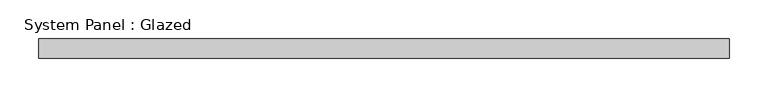
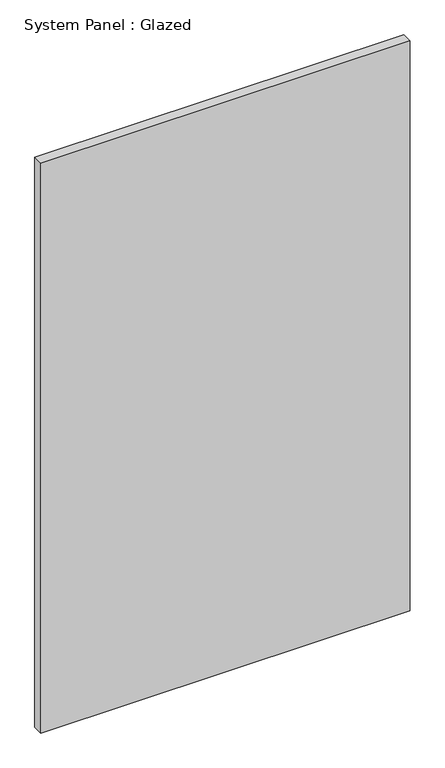
"""IFC4 building model written with IfcOpenShell, lengths in millimetres: plate geometry, System Panel : Glazed."""

from ifc_helpers import new_model, si_unit, origin, origin_with_axes, place, context, project, spatial, polyline, outline, extrude, source, transform, mapped, element, save


def system_panel_glazed_149319f3(model_context):
    return source(origin(), model_context, "Body", "SweptSolid", [
        extrude(outline(polyline([(447.675, 19.05), (-447.675, 19.05), (-447.675, 44.45), (447.675, 44.45), (447.675, 19.05)])), origin_with_axes(), (0.0, 0.0, 1.0), 1460.5),
    ])


if __name__ == "__main__":
    model = new_model("IFC4")
    model_context = context("Model", 3, world=origin())
    ifc_project = project(units=[si_unit("LENGTHUNIT", "METRE", prefix="MILLI")], contexts=[model_context])
    site = spatial("IfcSite", under=ifc_project)
    building = spatial("IfcBuilding", under=site)
    placement = place(None, origin())
    system_panel_glazed_shape = system_panel_glazed_149319f3(model_context)
    element("IfcPlate", 1, ObjectType="System Panel : Glazed", at=placement, inside=building, context=model_context, shape_type="MappedRepresentation", body=[
        mapped(system_panel_glazed_shape, transform((0.0, 0.0, 0.0), x_axis=(1.0, 0.0, 0.0), y_axis=(0.0, 1.0, 0.0), z_axis=(0.0, 0.0, 1.0))),
    ])
    save(model, "model.ifc")

# Revit data of these elements
# Type "System Panel : Glazed"
#   Construction Type Id = "GSP4R"
#   Analytic Construction = "1/8 in Pilkington single glazing"
#   Visual Light Transmittance = 0.9
#   Solar Heat Gain Coefficient = 0.86
#   Heat Transfer Coefficient (U) = 1.18115 BTU/(h·ft²·°F)
#   Define Thermal Properties by = 1
# Element 1 (IfcPlate, "System Panel : Glazed")
#   Materials on its faces: "Glass"
# Materials
#   "Glass": class "Glass", colour RGB 0 128 192, transparency 0.75, Description = "Soda Lime Glass", Cost = 0
